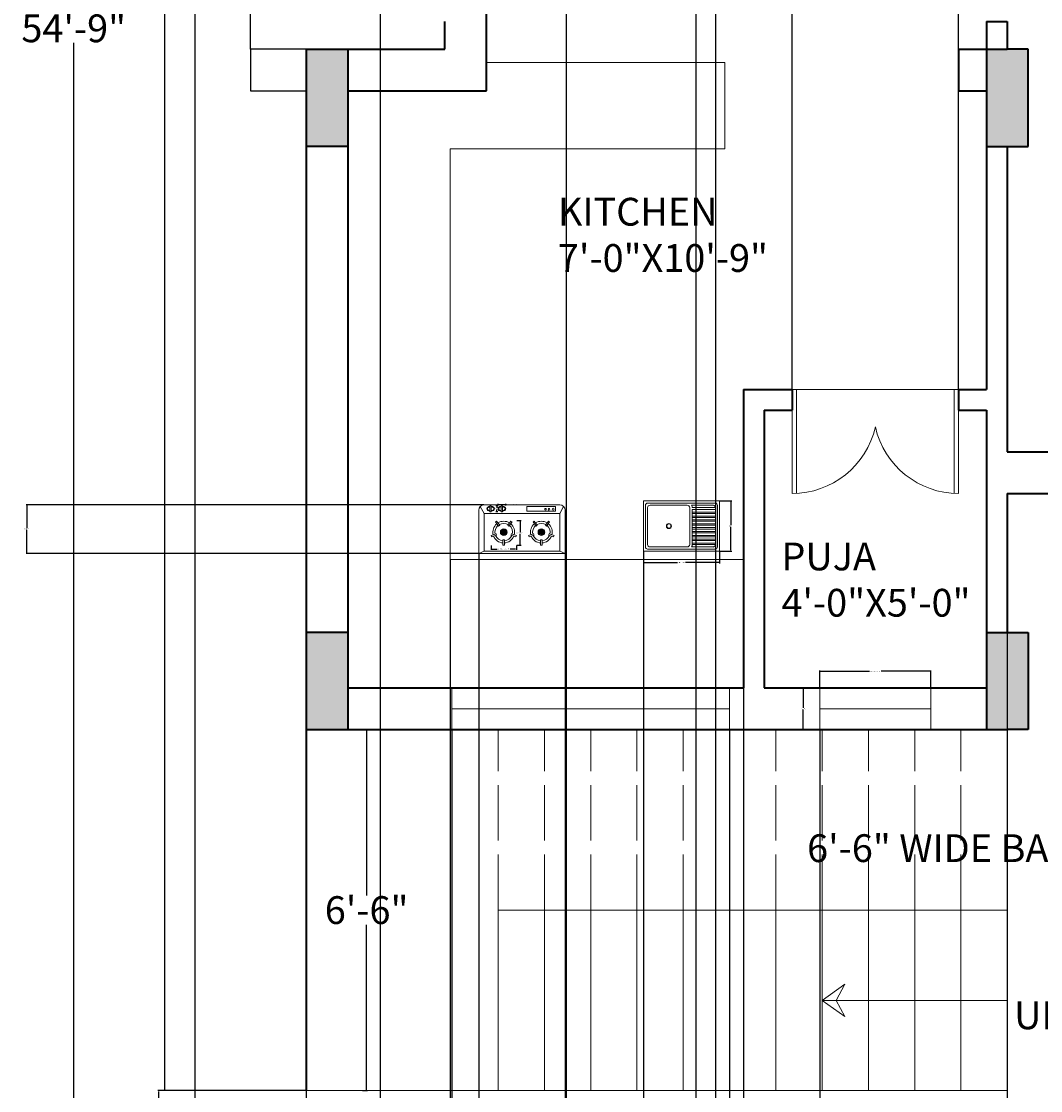
# Model space of a CAD drawing. Units: inches. Extents: x -36 to 401, y -686 to 73.
# Tile 2 of 15: x -36 to 184, y -550 to -319. Entities that reach past the tile are written whole.
import ezdxf

# ---------------------------------------------------------------- set-up
doc = ezdxf.new("R2010")
doc.units = ezdxf.units.IN
doc.header["$MEASUREMENT"] = 0
doc.linetypes.add('ACAD_ISO02W100', pattern=[15, 12, -3])
for name, color, linetype, lineweight in [('A-ANNO-DIMS', 2, 'Continuous', 18), ('A-ANNO-SYMB', 7, 'Continuous', 18), ('A-ANNO-TEXT', 7, 'Continuous', 18), ('A-AREA-IDEN', 7, 'Continuous', 18), ('A-COLS', 7, 'Continuous', 40), ('A-COLS-PATT', 22, 'Continuous', 13), ('A-DOOR', 3, 'Continuous', 18), ('A-EQPM', 8, 'Continuous', 13), ('A-FLOR', 7, 'Continuous', 25), ('A-FLOR-CASE', 9, 'Continuous', 18), ('A-FLOR-FIXT', 9, 'Continuous', 18), ('A-FLOR-OVHD', 8, 'ACAD_ISO02W100', 18), ('A-FLOR-STRS', 7, 'Continuous', 18), ('A-FLOR-STRS-OVHD', 8, 'ACAD_ISO02W100', 13), ('A-GLAZ', 4, 'Continuous', 18), ('A-WALL', 7, 'Continuous', 35), ('C-PROP', 7, 'Continuous', 25)]:
    doc.layers.add(name, color=color, linetype=linetype, lineweight=lineweight)
doc.styles.get("Standard").update_dxf_attribs({"font": 'arial.ttf'})
doc.dimstyles.get("Standard").update_dxf_attribs({"dimtxt": 0.18, "dimasz": 0.18, "dimexe": 0.18, "dimexo": 0.0625, "dimgap": 0.09, "dimtad": 0, "dimtih": 1, "dimtoh": 1, "dimdec": 0, "dimzin": 0, "dimdsep": 46, "dimlunit": 3, "dimtxsty": 'Standard', "dimcen": 0.09, "dimadec": 0, "dimazin": 0, "dimtfac": 1, "dimtdec": 0, "dimtofl": 0, "dimtmove": 0, "dimatfit": 3, "dimfxl": 1, "dimtolj": 1, "dimtzin": 0, "dimarcsym": 0})

# ---------------------------------------------------------------- blocks, each defined once
blk = doc.blocks.new('М12 540х820')
for p, q in [((0, 540), (-820, 540)), ((-820, 540), (-820, 0)), ((-798, 495), (-798, 45)), ((-45, 517), (-775, 517)), ((-775, 468), (-775, 72)), ((-348, 495), (-748, 495)), ((-320, 468), (-320, 72)), ((-302, 495), (-65, 495)), ((-294, 468), (-294, 472)), ((-294, 468), (-45, 468)), ((-45, 470), (-45, 468)), ((-22, 45), (-22, 495)), ((0, 0), (0, 540)), ((-294, 447), (-45, 447)), ((-294, 420), (-294, 447)), ((-294, 420), (-45, 420)), ((-294, 405), (-45, 405)), ((-294, 378), (-294, 405)), ((-294, 378), (-45, 378)), ((-294, 336), (-294, 363)), ((-294, 363), (-45, 363)), ((-45, 420), (-45, 447)), ((-45, 378), (-45, 405)), ((-45, 336), (-45, 363)), ((-294, 336), (-45, 336)), ((-294, 295), (-294, 322)), ((-294, 322), (-45, 322)), ((-294, 295), (-45, 295)), ((-294, 253), (-294, 280)), ((-294, 280), (-45, 280)), ((-294, 253), (-45, 253)), ((-294, 211), (-294, 238)), ((-294, 238), (-45, 238)), ((-45, 295), (-45, 322)), ((-45, 253), (-45, 280)), ((-45, 211), (-45, 238)), ((-294, 211), (-45, 211)), ((-294, 170), (-294, 197)), ((-294, 197), (-45, 197)), ((-294, 170), (-45, 170)), ((-294, 128), (-294, 155)), ((-294, 155), (-45, 155)), ((-294, 128), (-45, 128)), ((-45, 170), (-45, 197)), ((-45, 128), (-45, 155)), ((-820, 0), (0, 0)), ((-775, 22), (-45, 22)), ((-748, 45), (-348, 45)), ((-302, 45), (-65, 45)), ((-294, 114), (-45, 114)), ((-294, 87), (-294, 114)), ((-294, 87), (-45, 87)), ((-294, 72), (-45, 72)), ((-45, 87), (-45, 114)), ((-45, 70), (-45, 72))]:
    blk.add_line(p, q)
at = {"ltscale": 0.06}
for p, q in [((-820, 0), (-820, 540)), ((-820, 540), (0, 540)), ((0, 540), (0, 537)), ((0, 537), (0, 0)), ((-294, 447), (-45, 447)), ((-294, 405), (-294, 447)), ((-294, 363), (-294, 405)), ((-294, 322), (-294, 363)), ((-45, 447), (-45, 420)), ((-45, 420), (-45, 378)), ((-45, 378), (-45, 336)), ((-294, 280), (-294, 322)), ((-294, 238), (-294, 280)), ((-294, 197), (-294, 238)), ((-45, 336), (-45, 295)), ((-45, 295), (-45, 253)), ((-45, 253), (-45, 211)), ((-294, 155), (-294, 197)), ((-294, 114), (-294, 155)), ((-45, 211), (-45, 170)), ((-45, 170), (-45, 128)), ((-45, 128), (-45, 87)), ((0, 0), (-820, 0)), ((-294, 72), (-294, 114)), ((-45, 72), (-294, 72)), ((-45, 87), (-45, 72))]:
    blk.add_line(p, q, dxfattribs=at)
at = {"extrusion": (0, 0, -1)}
for centre, major_axis, start_param, end_param in [((-775, 495), (-15.9, 15.9), -0.785398, 0.785398), ((-775, 495), (-15.9, 15.9), -0.785398, 0.785398), ((-748, 468), (-19.1, -19.1), 0.785398, 2.356194), ((-748, 468), (-19.1, -19.1), 0.785398, 2.356194), ((-348, 468), (-19.1, 19.1), 0.785398, 2.356194), ((-348, 468), (-19.1, 19.1), 0.785398, 2.356194), ((-343, 468), (-35, 35), 1.779263, 2.356194), ((-343, 468), (-35, 35), 1.779263, 2.356192), ((-343, 468), (-35, 35), 2.356192, 2.356194), ((-72, 469), (-19.3, 19.3), 1.0328, 2.38382), ((-72, 469), (-19.3, 19.3), 1.0328, 1.064673), ((-72, 469), (-19.3, 19.3), 1.064673, 2.328569), ((-45, 495), (-15.9, -15.9), 2.356194, 3.926991), ((-45, 495), (-15.9, -15.9), 2.356194, 3.926991), ((-72, 469), (-19.3, 19.3), 2.328569, 2.38382), ((-545, 270), (-19.1, -19.1), 3.926991, 10.210176), ((-545, 270), (-19.1, -19.1), 3.926991, 10.210176), ((-545, 270), (-15.9, -15.9), 3.926991, 10.210176), ((-545, 270), (-15.9, -15.9), 3.926991, 10.210176), ((-775, 45), (-15.9, -15.9), 5.497787, 7.068583), ((-775, 45), (-15.9, -15.9), 5.497787, 7.068583), ((-748, 72), (-19.1, 19.1), 3.926991, 5.497787), ((-748, 72), (-19.1, 19.1), 3.926991, 5.497787), ((-348, 72), (-19.1, -19.1), 3.926991, 5.497787), ((-348, 72), (-19.1, -19.1), 3.926991, 5.497787), ((-343, 72), (-35, -35), 3.926991, 4.503922), ((-343, 72), (-35, -35), 3.926991, 4.503922), ((-72, 71), (-19.3, -19.3), 3.899365, 5.250385), ((-72, 71), (-19.3, -19.3), 5.218512, 5.250385), ((-72, 71), (-19.3, -19.3), 3.954617, 5.218512), ((-72, 71), (-19.3, -19.3), 3.899365, 3.954617), ((-45, 45), (-15.9, 15.9), 2.356194, 3.926991), ((-45, 45), (-15.9, 15.9), 2.356194, 3.926991)]:
    blk.add_ellipse(centre, major_axis=major_axis, ratio=1, start_param=start_param, end_param=end_param, dxfattribs=at)
blk = doc.blocks.new('*D2')
at = {"layer": 'A-ANNO-DIMS', "color": 0, "lineweight": -2, "transparency": 16777216}
for p, q in [((37.9, -472.21), (38.96, -472.21)), ((38.78, -472.39), (38.78, -508.06)), ((38.78, -550.03), (38.78, -514.36)), ((37.9, -550.21), (38.96, -550.21))]:
    blk.add_line(p, q, dxfattribs=at)
at = {"layer": 'A-ANNO-DIMS', "color": 0, "transparency": 16777216}
for points in [[(38.75, -472.39), (38.81, -472.39), (38.78, -472.21)], [(38.75, -550.03), (38.81, -550.03), (38.78, -550.21)]]:
    blk.add_solid(points, dxfattribs=at)
at = {"layer": 'Defpoints', "color": 0, "transparency": 16777216}
for p in [(37.84, -472.21), (38.78, -472.21), (37.84, -550.21)]:
    blk.add_point(p, dxfattribs=at)
at = {"layer": 'A-ANNO-DIMS', "color": 0, "transparency": 16777216, "insert": (38.78, -511.21), "char_height": 6, "attachment_point": 5}
blk.add_mtext('\\A1;6\'-6"', dxfattribs=at)
blk = doc.blocks.new('*D8')
at = {"layer": 'A-ANNO-DIMS', "color": 0, "lineweight": -2, "transparency": 16777216}
for p, q in [((25.63, 7.79), (-24.68, 7.79)), ((-24.5, 7.61), (-24.5, -317.56)), ((-24.5, -649.03), (-24.5, -323.86)), ((1.63, -649.21), (-24.68, -649.21))]:
    blk.add_line(p, q, dxfattribs=at)
at = {"layer": 'A-ANNO-DIMS', "color": 0, "transparency": 16777216}
for points in [[(-24.53, 7.61), (-24.47, 7.61), (-24.5, 7.79)], [(-24.53, -649.03), (-24.47, -649.03), (-24.5, -649.21)]]:
    blk.add_solid(points, dxfattribs=at)
at = {"layer": 'Defpoints', "color": 0, "transparency": 16777216}
for p in [(25.69, 7.79), (-24.5, -649.21), (1.69, -649.21)]:
    blk.add_point(p, dxfattribs=at)
at = {"layer": 'A-ANNO-DIMS', "color": 0, "transparency": 16777216, "insert": (-24.5, -320.71), "char_height": 6, "attachment_point": 5}
blk.add_mtext('\\A1;54\'-9"', dxfattribs=at)
blk = doc.blocks.new('*D11')
at = {"layer": 'A-ANNO-DIMS', "color": 0, "lineweight": -2, "transparency": 16777216}
for p, q in [((25.63, 7.79), (-5.02, 7.79)), ((-4.84, 7.61), (-4.84, -268.06)), ((-4.84, -550.03), (-4.84, -274.36)), ((25.63, -550.21), (-5.02, -550.21))]:
    blk.add_line(p, q, dxfattribs=at)
at = {"layer": 'A-ANNO-DIMS', "color": 0, "transparency": 16777216}
for points in [[(-4.87, 7.61), (-4.81, 7.61), (-4.84, 7.79)], [(-4.87, -550.03), (-4.81, -550.03), (-4.84, -550.21)]]:
    blk.add_solid(points, dxfattribs=at)
at = {"layer": 'Defpoints', "color": 0, "transparency": 16777216}
for p in [(25.69, 7.79), (-4.84, -550.21), (25.69, -550.21)]:
    blk.add_point(p, dxfattribs=at)
at = {"layer": 'A-ANNO-DIMS', "color": 0, "transparency": 16777216, "insert": (-4.84, -271.21), "char_height": 6, "attachment_point": 5}
blk.add_mtext('\\A1;46\'-6"', dxfattribs=at)
blk = doc.blocks.new('*D12')
at = {"layer": 'A-ANNO-DIMS', "color": 0, "lineweight": -2, "transparency": 16777216}
for p, q in [((25.63, -550.21), (-6.34, -550.21)), ((-6.16, -550.39), (-6.16, -596.55)), ((-6.16, -649.03), (-6.16, -602.87)), ((25.63, -649.21), (-6.34, -649.21))]:
    blk.add_line(p, q, dxfattribs=at)
at = {"layer": 'A-ANNO-DIMS', "color": 0, "transparency": 16777216}
for points in [[(-6.19, -550.39), (-6.13, -550.39), (-6.16, -550.21)], [(-6.19, -649.03), (-6.13, -649.03), (-6.16, -649.21)]]:
    blk.add_solid(points, dxfattribs=at)
at = {"layer": 'Defpoints', "color": 0, "transparency": 16777216}
for p in [(25.69, -550.21), (-6.16, -649.21), (25.69, -649.21)]:
    blk.add_point(p, dxfattribs=at)
at = {"layer": 'A-ANNO-DIMS', "color": 0, "transparency": 16777216, "insert": (-6.16, -599.71), "char_height": 6, "attachment_point": 5}
blk.add_mtext('\\A1;8\'-3"', dxfattribs=at)
blk = doc.blocks.new('WIN-24IN')
for p, q in [((0, 9), (24, 9)), ((0, 0), (0, 9)), ((24, 9), (24, 0)), ((0, 4.5), (24, 4.5)), ((24, 0), (0, 0))]:
    blk.add_line(p, q)
blk = doc.blocks.new('WIN-60IN')
for p, q in [((0, 9), (60, 9)), ((0, 0), (0, 9)), ((60, 9), (60, 0)), ((0, 4.5), (60, 4.5)), ((60, 0), (0, 0))]:
    blk.add_line(p, q)
blk = doc.blocks.new('HOB-BURNER')
for p, q in [((0.95, 5.03), (1.21, 5.22)), ((1.62, 4.11), (0.95, 5.03)), ((1.21, 5.22), (1.87, 4.3)), ((3.61, 4.3), (4.28, 5.22)), ((4.54, 5.03), (3.87, 4.11)), ((4.28, 5.22), (4.54, 5.03)), ((0, 2.11), (1.08, 2.46)), ((1.08, 2.46), (1.18, 2.16)), ((1.87, 4.3), (1.62, 4.11)), ((2.74, 2.83), (2.02, 2.83)), ((2.74, 2.83), (2.06, 3.05)), ((2.74, 2.83), (2.06, 2.61)), ((2.74, 2.83), (2.16, 3.25)), ((2.74, 2.83), (2.16, 2.41)), ((2.74, 2.83), (2.32, 3.41)), ((2.74, 2.83), (2.32, 2.25)), ((2.74, 2.83), (2.52, 3.51)), ((2.74, 2.83), (2.52, 2.15)), ((2.74, 2.83), (2.74, 3.55)), ((2.74, 2.83), (2.97, 3.51)), ((2.74, 2.83), (3.17, 3.41)), ((2.74, 2.83), (3.32, 3.25)), ((2.74, 2.83), (3.43, 3.05)), ((2.74, 2.83), (3.46, 2.83)), ((2.74, 2.83), (3.43, 2.61)), ((2.74, 2.83), (3.32, 2.41)), ((2.74, 2.83), (3.17, 2.25)), ((2.74, 2.83), (2.97, 2.15)), ((2.74, 2.83), (2.74, 2.11)), ((3.87, 4.11), (3.61, 4.3)), ((4.31, 2.16), (4.41, 2.46)), ((4.41, 2.46), (5.49, 2.11)), ((0.1, 1.81), (0, 2.11)), ((1.18, 2.16), (0.1, 1.81)), ((2.58, 1.13), (2.9, 1.13)), ((2.58, 0), (2.58, 1.13)), ((2.9, 1.13), (2.9, 0)), ((5.39, 1.81), (4.31, 2.16)), ((5.49, 2.11), (5.39, 1.81)), ((2.9, 0), (2.58, 0))]:
    blk.add_line(p, q)
blk.add_circle((2.74, 2.83), 0.721)
for radius, start, end in [(2.35, 129.8765, 194.1235), (2.35, 57.8765, 122.1235), (1.89, 58.8365, 121.1635), (2.35, 345.8765, 50.1235), (1.89, 130.8365, 193.1635), (1.89, 346.8365, 49.1635), (2.35, 201.8765, 266.1235), (1.89, 202.8365, 265.1635), (1.89, 274.8365, 337.1635), (2.35, 273.8765, 338.1235)]:
    blk.add_arc((2.74, 2.83), radius, start, end)
blk = doc.blocks.new('HOB-CONTROL')
for p, q in [((0.67, 0), (0.67, 1.29)), ((0.67, 1.29), (0.97, 1.29)), ((0.97, 1.29), (0.97, 0)), ((0.97, 0), (0.67, 0))]:
    blk.add_line(p, q)
for major_axis, start_param, end_param in [((0.835, 0), 1.774361, 4.508825), ((-0.835, 0), 1.73081, 4.552375)]:
    blk.add_ellipse((0.84, 0.65), major_axis=major_axis, ratio=0.671641, start_param=start_param, end_param=end_param)
for points, knots in [([(0.67, 1.08), (0.63, 1.08), (0.59, 1.07), (0.5, 1.04), (0.45, 1.03), (0.36, 0.98), (0.32, 0.96), (0.25, 0.91), (0.23, 0.88), (0.18, 0.83), (0.16, 0.8), (0.13, 0.74), (0.12, 0.71), (0.12, 0.66), (0.12, 0.63), (0.13, 0.57), (0.14, 0.54), (0.17, 0.49), (0.19, 0.46), (0.24, 0.4), (0.27, 0.38), (0.35, 0.33), (0.39, 0.31), (0.48, 0.27), (0.52, 0.25), (0.61, 0.23), (0.64, 0.22), (0.67, 0.22)], [8.079302, 8.079302, 8.079302, 8.079302, 8.245651, 8.245651, 8.463703, 8.463703, 8.681755, 8.681755, 8.899807, 8.899807, 9.117859, 9.117859, 9.33591, 9.33591, 9.553962, 9.553962, 9.772014, 9.772014, 9.990066, 9.990066, 10.208118, 10.208118, 10.426169, 10.426169, 10.644221, 10.644221, 10.770253, 10.770253, 10.770253, 10.770253]), ([(0.97, 0.21), (1, 0.22), (1.03, 0.22), (1.11, 0.24), (1.16, 0.26), (1.25, 0.29), (1.3, 0.31), (1.37, 0.36), (1.41, 0.39), (1.47, 0.44), (1.49, 0.47), (1.52, 0.52), (1.54, 0.55), (1.55, 0.61), (1.55, 0.63), (1.55, 0.65), (1.55, 0.68), (1.55, 0.71), (1.53, 0.76), (1.52, 0.79), (1.48, 0.85), (1.45, 0.88), (1.39, 0.93), (1.35, 0.96), (1.27, 1), (1.23, 1.02), (1.13, 1.05), (1.08, 1.07), (1.01, 1.08), (0.99, 1.08), (0.97, 1.09)], [4.889299, 4.889299, 4.889299, 4.889299, 5.015191, 5.015191, 5.233243, 5.233243, 5.451295, 5.451295, 5.669347, 5.669347, 5.887399, 5.887399, 6.10545, 6.10545, 6.283185, 6.283185, 6.283185, 6.501237, 6.501237, 6.719289, 6.719289, 6.937341, 6.937341, 7.155392, 7.155392, 7.373444, 7.373444, 7.591496, 7.591496, 7.677072, 7.677072, 7.677072, 7.677072])]:
    blk.add_open_spline(points, degree=3, knots=knots)
blk = doc.blocks.new('*D39')
at = {"layer": 'A-ANNO-DIMS', "color": 0, "lineweight": -2, "transparency": 16777216}
for p, q in [((136.69, -463.15), (136.69, -459.43)), ((136.87, -459.61), (147.46, -459.61)), ((160.51, -459.61), (149.92, -459.61)), ((160.69, -463.15), (160.69, -459.43))]:
    blk.add_line(p, q, dxfattribs=at)
at = {"layer": 'A-ANNO-DIMS', "color": 0, "transparency": 16777216}
for points in [[(136.87, -459.58), (136.87, -459.64), (136.69, -459.61)], [(160.51, -459.58), (160.51, -459.64), (160.69, -459.61)]]:
    blk.add_solid(points, dxfattribs=at)
at = {"layer": 'Defpoints', "color": 0, "transparency": 16777216}
for p in [(160.69, -459.61), (136.69, -463.21), (160.69, -463.21)]:
    blk.add_point(p, dxfattribs=at)
at = {"layer": 'A-ANNO-DIMS', "color": 0, "transparency": 16777216, "insert": (148.69, -459.61), "char_height": 0.18, "attachment_point": 5}
blk.add_mtext('\\A1;WINDOW 2\'-0" TYP.', dxfattribs=at)
blk = doc.blocks.new('*D40')
at = {"layer": 'A-ANNO-DIMS', "color": 0, "lineweight": -2, "transparency": 16777216}
for p, q in [((136.63, -463.21), (132.91, -463.21)), ((133.09, -463.39), (133.09, -467.53)), ((133.09, -472.03), (133.09, -467.89)), ((136.63, -472.21), (132.91, -472.21))]:
    blk.add_line(p, q, dxfattribs=at)
at = {"layer": 'A-ANNO-DIMS', "color": 0, "transparency": 16777216}
for points in [[(133.06, -463.39), (133.12, -463.39), (133.09, -463.21)], [(133.06, -472.03), (133.12, -472.03), (133.09, -472.21)]]:
    blk.add_solid(points, dxfattribs=at)
at = {"layer": 'Defpoints', "color": 0, "transparency": 16777216}
for p in [(133.09, -463.21), (136.69, -463.21), (136.69, -472.21)]:
    blk.add_point(p, dxfattribs=at)
at = {"layer": 'A-ANNO-DIMS', "color": 0, "transparency": 16777216, "insert": (133.09, -467.71), "char_height": 0.18, "attachment_point": 5}
blk.add_mtext('\\A1;0\'-9" TYP.', dxfattribs=at)
blk = doc.blocks.new('*D53')
at = {"layer": 'A-ANNO-DIMS', "color": 0, "lineweight": -2, "transparency": 16777216}
for p, q in [((65.66, -432.44), (65.66, -433.38)), ((65.84, -433.2), (67, -433.2)), ((70.97, -433.2), (69.82, -433.2)), ((71.15, -432.44), (71.15, -433.38))]:
    blk.add_line(p, q, dxfattribs=at)
at = {"layer": 'A-ANNO-DIMS', "color": 0, "transparency": 16777216}
for points in [[(65.84, -433.17), (65.84, -433.23), (65.66, -433.2)], [(70.97, -433.17), (70.97, -433.23), (71.15, -433.2)]]:
    blk.add_solid(points, dxfattribs=at)
at = {"layer": 'Defpoints', "color": 0, "transparency": 16777216}
for p in [(65.66, -432.38), (71.15, -432.38), (71.15, -433.2)]:
    blk.add_point(p, dxfattribs=at)
at = {"layer": 'A-ANNO-DIMS', "color": 0, "transparency": 16777216, "insert": (68.41, -433.2), "char_height": 0.18, "attachment_point": 5}
blk.add_mtext('\\A1;BURNER 0\'-5 1/2" TYP.', dxfattribs=at)
blk = doc.blocks.new('*D54')
at = {"layer": 'A-ANNO-DIMS', "color": 0, "lineweight": -2, "transparency": 16777216}
for p, q in [((71.21, -427.07), (72.15, -427.07)), ((71.97, -427.25), (71.97, -429.54)), ((71.97, -432.2), (71.97, -429.91)), ((71.21, -432.38), (72.15, -432.38))]:
    blk.add_line(p, q, dxfattribs=at)
at = {"layer": 'A-ANNO-DIMS', "color": 0, "transparency": 16777216}
for points in [[(71.94, -427.25), (72, -427.25), (71.97, -427.07)], [(71.94, -432.2), (72, -432.2), (71.97, -432.38)]]:
    blk.add_solid(points, dxfattribs=at)
at = {"layer": 'Defpoints', "color": 0, "transparency": 16777216}
for p in [(71.15, -427.07), (71.97, -427.07), (71.15, -432.38)]:
    blk.add_point(p, dxfattribs=at)
at = {"layer": 'A-ANNO-DIMS', "color": 0, "transparency": 16777216, "insert": (71.97, -429.73), "char_height": 0.18, "attachment_point": 5}
blk.add_mtext('\\A1;0\'-5 1/2" TYP.', dxfattribs=at)
blk = doc.blocks.new('*D55')
at = {"layer": 'A-ANNO-DIMS', "color": 0, "lineweight": -2, "transparency": 16777216}
for p, q in [((67.17, -423.79), (67.17, -423.43)), ((67.35, -423.61), (68.65, -423.61)), ((68.83, -423.79), (68.83, -423.43)), ((68.83, -423.61), (69.01, -423.61))]:
    blk.add_line(p, q, dxfattribs=at)
at = {"layer": 'A-ANNO-DIMS', "color": 0, "transparency": 16777216}
for points in [[(67.35, -423.58), (67.35, -423.64), (67.17, -423.61)], [(68.65, -423.58), (68.65, -423.64), (68.83, -423.61)]]:
    blk.add_solid(points, dxfattribs=at)
at = {"layer": 'Defpoints', "color": 0, "transparency": 16777216}
for p in [(67.17, -423.86), (68.83, -423.61), (68.83, -423.86)]:
    blk.add_point(p, dxfattribs=at)
at = {"layer": 'A-ANNO-DIMS', "color": 0, "transparency": 16777216, "insert": (70.51, -423.61), "char_height": 0.18, "attachment_point": 5}
blk.add_mtext('\\A1;CONTROL 0\'-1 1/2" TYP.', dxfattribs=at)
blk = doc.blocks.new('*D56')
at = {"layer": 'A-ANNO-DIMS', "color": 0, "lineweight": -2, "transparency": 16777216}
for p, q in [((67.1, -423.86), (66.73, -423.86)), ((66.91, -424.04), (66.91, -424.32)), ((66.91, -424.97), (66.91, -424.69)), ((67.1, -425.15), (66.73, -425.15))]:
    blk.add_line(p, q, dxfattribs=at)
at = {"layer": 'A-ANNO-DIMS', "color": 0, "transparency": 16777216}
for points in [[(66.88, -424.04), (66.94, -424.04), (66.91, -423.86)], [(66.88, -424.97), (66.94, -424.97), (66.91, -425.15)]]:
    blk.add_solid(points, dxfattribs=at)
at = {"layer": 'Defpoints', "color": 0, "transparency": 16777216}
for p in [(66.91, -423.86), (67.17, -423.86), (67.17, -425.15)]:
    blk.add_point(p, dxfattribs=at)
at = {"layer": 'A-ANNO-DIMS', "color": 0, "transparency": 16777216, "insert": (66.91, -424.5), "char_height": 0.18, "attachment_point": 5}
blk.add_mtext('\\A1;0\'-1 1/2" TYP.', dxfattribs=at)
blk = doc.blocks.new('*D61')
at = {"layer": 'A-ANNO-DIMS', "color": 0, "lineweight": -2, "transparency": 16777216}
for p, q in [((98.57, -433.72), (98.57, -436.31)), ((115.03, -433.72), (115.03, -436.31)), ((98.75, -436.13), (105.93, -436.13)), ((114.85, -436.13), (107.66, -436.13))]:
    blk.add_line(p, q, dxfattribs=at)
at = {"layer": 'A-ANNO-DIMS', "color": 0, "transparency": 16777216}
for points in [[(98.75, -436.1), (98.75, -436.16), (98.57, -436.13)], [(114.85, -436.1), (114.85, -436.16), (115.03, -436.13)]]:
    blk.add_solid(points, dxfattribs=at)
at = {"layer": 'Defpoints', "color": 0, "transparency": 16777216}
for p in [(98.57, -433.66), (115.03, -433.66), (115.03, -436.13)]:
    blk.add_point(p, dxfattribs=at)
at = {"layer": 'A-ANNO-DIMS', "color": 0, "transparency": 16777216, "insert": (106.8, -436.13), "char_height": 0.18, "attachment_point": 5}
blk.add_mtext('\\A1;SINK 1\'-4 1/2"', dxfattribs=at)
blk = doc.blocks.new('*D62')
at = {"layer": 'A-ANNO-DIMS', "color": 0, "lineweight": -2, "transparency": 16777216}
for p, q in [((115.09, -422.82), (117.67, -422.82)), ((117.49, -423), (117.49, -428.06)), ((117.49, -433.48), (117.49, -428.42)), ((115.09, -433.66), (117.67, -433.66))]:
    blk.add_line(p, q, dxfattribs=at)
at = {"layer": 'A-ANNO-DIMS', "color": 0, "transparency": 16777216}
for points in [[(117.46, -423), (117.52, -423), (117.49, -422.82)], [(117.46, -433.48), (117.52, -433.48), (117.49, -433.66)]]:
    blk.add_solid(points, dxfattribs=at)
at = {"layer": 'Defpoints', "color": 0, "transparency": 16777216}
for p in [(115.03, -422.82), (117.49, -422.82), (115.03, -433.66)]:
    blk.add_point(p, dxfattribs=at)
at = {"layer": 'A-ANNO-DIMS', "color": 0, "transparency": 16777216, "insert": (117.49, -428.24), "char_height": 0.18, "attachment_point": 5}
blk.add_mtext('\\A1;0\'-11"', dxfattribs=at)
blk = doc.blocks.new('*D73')
at = {"layer": 'A-ANNO-DIMS', "color": 0, "lineweight": -2, "transparency": 16777216}
for p, q in [((177.19, -421.27), (177.19, -685.69)), ((253.69, -421.27), (253.69, -685.69)), ((177.37, -685.51), (214.9, -685.51)), ((253.51, -685.51), (215.98, -685.51))]:
    blk.add_line(p, q, dxfattribs=at)
at = {"layer": 'A-ANNO-DIMS', "color": 0, "transparency": 16777216}
for points in [[(177.37, -685.48), (177.37, -685.54), (177.19, -685.51)], [(253.51, -685.48), (253.51, -685.54), (253.69, -685.51)]]:
    blk.add_solid(points, dxfattribs=at)
at = {"layer": 'Defpoints', "color": 0, "transparency": 16777216}
for p in [(177.19, -421.21), (253.69, -421.21), (253.69, -685.51)]:
    blk.add_point(p, dxfattribs=at)
at = {"layer": 'A-ANNO-DIMS', "color": 0, "transparency": 16777216, "insert": (215.44, -685.51), "char_height": 0.18, "attachment_point": 5}
blk.add_mtext('\\A1;6\'-4 1/2"', dxfattribs=at)
blk = doc.blocks.new('*D75')
at = {"layer": 'A-ANNO-DIMS', "color": 0, "lineweight": -2, "transparency": 16777216}
for p, q in [((25.69, -472.27), (25.69, -685.69)), ((57.17, -472.27), (57.17, -685.69)), ((25.87, -685.51), (40.89, -685.51)), ((56.99, -685.51), (41.97, -685.51))]:
    blk.add_line(p, q, dxfattribs=at)
at = {"layer": 'A-ANNO-DIMS', "color": 0, "transparency": 16777216}
for points in [[(25.87, -685.48), (25.87, -685.54), (25.69, -685.51)], [(56.99, -685.48), (56.99, -685.54), (57.17, -685.51)]]:
    blk.add_solid(points, dxfattribs=at)
at = {"layer": 'Defpoints', "color": 0, "transparency": 16777216}
for p in [(25.69, -472.21), (57.17, -472.21), (57.17, -685.51)]:
    blk.add_point(p, dxfattribs=at)
at = {"layer": 'A-ANNO-DIMS', "color": 0, "transparency": 16777216, "insert": (41.43, -685.51), "char_height": 0.18, "attachment_point": 5}
blk.add_mtext('\\A1;2\'-7 1/2"', dxfattribs=at)
blk = doc.blocks.new('*D76')
at = {"layer": 'A-ANNO-DIMS', "color": 0, "lineweight": -2, "transparency": 16777216}
for p, q in [((117.19, -472.27), (117.19, -685.69)), ((136.69, -472.27), (136.69, -685.69)), ((117.37, -685.51), (126.41, -685.51)), ((136.51, -685.51), (127.47, -685.51))]:
    blk.add_line(p, q, dxfattribs=at)
at = {"layer": 'A-ANNO-DIMS', "color": 0, "transparency": 16777216}
for points in [[(117.37, -685.48), (117.37, -685.54), (117.19, -685.51)], [(136.51, -685.48), (136.51, -685.54), (136.69, -685.51)]]:
    blk.add_solid(points, dxfattribs=at)
at = {"layer": 'Defpoints', "color": 0, "transparency": 16777216}
for p in [(117.19, -472.21), (136.69, -472.21), (136.69, -685.51)]:
    blk.add_point(p, dxfattribs=at)
at = {"layer": 'A-ANNO-DIMS', "color": 0, "transparency": 16777216, "insert": (126.94, -685.51), "char_height": 0.18, "attachment_point": 5}
blk.add_mtext('\\A1;1\'-7 1/2"', dxfattribs=at)
blk = doc.blocks.new('*D79')
at = {"layer": 'A-ANNO-DIMS', "color": 0, "lineweight": -2, "transparency": 16777216}
for p, q in [((130.69, -398.65), (130.69, 68.27)), ((130.87, 68.09), (148.36, 68.09)), ((166.51, 68.09), (149.02, 68.09)), ((166.69, -398.65), (166.69, 68.27))]:
    blk.add_line(p, q, dxfattribs=at)
at = {"layer": 'A-ANNO-DIMS', "color": 0, "transparency": 16777216}
for points in [[(130.87, 68.12), (130.87, 68.06), (130.69, 68.09)], [(166.51, 68.12), (166.51, 68.06), (166.69, 68.09)]]:
    blk.add_solid(points, dxfattribs=at)
at = {"layer": 'Defpoints', "color": 0, "transparency": 16777216}
for p in [(166.69, 68.09), (130.69, -398.71), (166.69, -398.71)]:
    blk.add_point(p, dxfattribs=at)
at = {"layer": 'A-ANNO-DIMS', "color": 0, "transparency": 16777216, "insert": (148.69, 68.09), "char_height": 0.18, "attachment_point": 5}
blk.add_mtext('\\A1;3\'-0"', dxfattribs=at)
blk = doc.blocks.new('*D80')
at = {"layer": 'A-ANNO-DIMS', "color": 0, "lineweight": -2, "transparency": 16777216}
for p, q in [((56.84, -435.52), (56.84, -685.69)), ((120.19, -435.52), (120.19, -685.69)), ((57.02, -685.51), (87.97, -685.51)), ((120.01, -685.51), (89.05, -685.51))]:
    blk.add_line(p, q, dxfattribs=at)
at = {"layer": 'A-ANNO-DIMS', "color": 0, "transparency": 16777216}
for points in [[(57.02, -685.48), (57.02, -685.54), (56.84, -685.51)], [(120.01, -685.48), (120.01, -685.54), (120.19, -685.51)]]:
    blk.add_solid(points, dxfattribs=at)
at = {"layer": 'Defpoints', "color": 0, "transparency": 16777216}
for p in [(56.84, -435.46), (120.19, -435.46), (120.19, -685.51)]:
    blk.add_point(p, dxfattribs=at)
at = {"layer": 'A-ANNO-DIMS', "color": 0, "transparency": 16777216, "insert": (88.51, -685.51), "char_height": 0.18, "attachment_point": 5}
blk.add_mtext('\\A1;5\'-3 1/2"', dxfattribs=at)
blk = doc.blocks.new('*D81')
at = {"layer": 'A-ANNO-DIMS', "color": 0, "lineweight": -2, "transparency": 16777216}
for p, q in [((63, -434.2), (63, -685.69)), ((81.66, -434.2), (81.66, -685.69)), ((63.18, -685.51), (71.8, -685.51)), ((81.48, -685.51), (72.86, -685.51))]:
    blk.add_line(p, q, dxfattribs=at)
at = {"layer": 'A-ANNO-DIMS', "color": 0, "transparency": 16777216}
for points in [[(63.18, -685.48), (63.18, -685.54), (63, -685.51)], [(81.48, -685.48), (81.48, -685.54), (81.66, -685.51)]]:
    blk.add_solid(points, dxfattribs=at)
at = {"layer": 'Defpoints', "color": 0, "transparency": 16777216}
for p in [(63, -434.14), (81.66, -434.14), (81.66, -685.51)]:
    blk.add_point(p, dxfattribs=at)
at = {"layer": 'A-ANNO-DIMS', "color": 0, "transparency": 16777216, "insert": (72.33, -685.51), "char_height": 0.18, "attachment_point": 5}
blk.add_mtext('\\A1;1\'-6 1/2"', dxfattribs=at)
blk = doc.blocks.new('*D82')
at = {"layer": 'A-ANNO-DIMS', "color": 0, "lineweight": -2, "transparency": 16777216}
for p, q in [((64.1, -423.65), (-34.79, -423.65)), ((-34.61, -423.83), (-34.61, -428.71)), ((-34.61, -433.96), (-34.61, -429.08)), ((62.94, -434.14), (-34.79, -434.14))]:
    blk.add_line(p, q, dxfattribs=at)
at = {"layer": 'A-ANNO-DIMS', "color": 0, "transparency": 16777216}
for points in [[(-34.64, -423.83), (-34.58, -423.83), (-34.61, -423.65)], [(-34.64, -433.96), (-34.58, -433.96), (-34.61, -434.14)]]:
    blk.add_solid(points, dxfattribs=at)
at = {"layer": 'Defpoints', "color": 0, "transparency": 16777216}
for p in [(64.17, -423.65), (-34.61, -434.14), (63, -434.14)]:
    blk.add_point(p, dxfattribs=at)
at = {"layer": 'A-ANNO-DIMS', "color": 0, "transparency": 16777216, "insert": (-34.61, -428.89), "char_height": 0.18, "attachment_point": 5}
blk.add_mtext('\\A1;0\'-10 1/2"', dxfattribs=at)
blk = doc.blocks.new('*D83')
at = {"layer": 'A-ANNO-DIMS', "color": 0, "lineweight": -2, "transparency": 16777216}
for p, q in [((63, -434.2), (63, -685.69)), ((56.84, -435.52), (56.84, -685.69)), ((57.02, -685.51), (59.59, -685.51)), ((62.82, -685.51), (60.25, -685.51))]:
    blk.add_line(p, q, dxfattribs=at)
at = {"layer": 'A-ANNO-DIMS', "color": 0, "transparency": 16777216}
for points in [[(57.02, -685.48), (57.02, -685.54), (56.84, -685.51)], [(62.82, -685.48), (62.82, -685.54), (63, -685.51)]]:
    blk.add_solid(points, dxfattribs=at)
at = {"layer": 'Defpoints', "color": 0, "transparency": 16777216}
for p in [(63, -434.14), (56.84, -435.46), (63, -685.51)]:
    blk.add_point(p, dxfattribs=at)
at = {"layer": 'A-ANNO-DIMS', "color": 0, "transparency": 16777216, "insert": (59.92, -685.51), "char_height": 0.18, "attachment_point": 5}
blk.add_mtext('\\A1;0\'-6"', dxfattribs=at)
blk = doc.blocks.new('*D84')
at = {"layer": 'A-ANNO-DIMS', "color": 0, "lineweight": -2, "transparency": 16777216}
for p, q in [((81.66, -434.2), (81.66, -685.69)), ((98.57, -433.72), (98.57, -685.69)), ((81.84, -685.51), (89.79, -685.51)), ((98.39, -685.51), (90.43, -685.51))]:
    blk.add_line(p, q, dxfattribs=at)
at = {"layer": 'A-ANNO-DIMS', "color": 0, "transparency": 16777216}
for points in [[(81.84, -685.48), (81.84, -685.54), (81.66, -685.51)], [(98.39, -685.48), (98.39, -685.54), (98.57, -685.51)]]:
    blk.add_solid(points, dxfattribs=at)
at = {"layer": 'Defpoints', "color": 0, "transparency": 16777216}
for p in [(81.66, -434.14), (98.57, -433.66), (98.57, -685.51)]:
    blk.add_point(p, dxfattribs=at)
at = {"layer": 'A-ANNO-DIMS', "color": 0, "transparency": 16777216, "insert": (90.11, -685.51), "char_height": 0.18, "attachment_point": 5}
blk.add_mtext('\\A1;1\'-5"', dxfattribs=at)
blk = doc.blocks.new('*D85')
at = {"layer": 'A-ANNO-DIMS', "color": 0, "lineweight": -2, "transparency": 16777216}
for p, q in [((114.18, -126.31), (114.18, -685.69)), ((41.7, -137.56), (41.7, -685.69)), ((41.88, -685.51), (77.4, -685.51)), ((114, -685.51), (78.48, -685.51))]:
    blk.add_line(p, q, dxfattribs=at)
at = {"layer": 'A-ANNO-DIMS', "color": 0, "transparency": 16777216}
for points in [[(41.88, -685.48), (41.88, -685.54), (41.7, -685.51)], [(114, -685.48), (114, -685.54), (114.18, -685.51)]]:
    blk.add_solid(points, dxfattribs=at)
at = {"layer": 'Defpoints', "color": 0, "transparency": 16777216}
for p in [(114.18, -126.25), (41.7, -137.5), (114.18, -685.51)]:
    blk.add_point(p, dxfattribs=at)
at = {"layer": 'A-ANNO-DIMS', "color": 0, "transparency": 16777216, "insert": (77.94, -685.51), "char_height": 0.18, "attachment_point": 5}
blk.add_mtext('\\A1;6\'-0 1/2"', dxfattribs=at)
blk = doc.blocks.new('*D89')
at = {"layer": 'A-ANNO-DIMS', "color": 0, "lineweight": -2, "transparency": 16777216}
for p, q in [((81.9, -256.42), (81.9, -685.69)), ((109.9, -256.42), (109.9, -685.69)), ((82.08, -685.51), (95.57, -685.51)), ((109.72, -685.51), (96.23, -685.51))]:
    blk.add_line(p, q, dxfattribs=at)
at = {"layer": 'A-ANNO-DIMS', "color": 0, "transparency": 16777216}
for points in [[(82.08, -685.48), (82.08, -685.54), (81.9, -685.51)], [(109.72, -685.48), (109.72, -685.54), (109.9, -685.51)]]:
    blk.add_solid(points, dxfattribs=at)
at = {"layer": 'Defpoints', "color": 0, "transparency": 16777216}
for p in [(81.9, -256.36), (109.9, -256.36), (109.9, -685.51)]:
    blk.add_point(p, dxfattribs=at)
at = {"layer": 'A-ANNO-DIMS', "color": 0, "transparency": 16777216, "insert": (95.9, -685.51), "char_height": 0.18, "attachment_point": 5}
blk.add_mtext('\\A1;2\'-4"', dxfattribs=at)

msp = doc.modelspace()

# ---------------------------------------------------------------- hatches: boundary and pattern name
at = {"layer": 'A-COLS-PATT'}
h = msp.add_hatch(color=256, dxfattribs=at)
h.dxf.hatch_style = 1
h.paths.add_polyline_path([(34.69, 7.79), (25.69, 7.79), (25.69, -13.21), (34.69, -13.21)])
h.paths.add_polyline_path([(172.69, -13.21), (177.19, -13.21), (181.69, -13.21), (181.69, 7.79), (172.69, 7.79)])
h.paths.add_polyline_path([(322.69, 7.79), (313.69, 7.79), (313.69, -13.21), (322.69, -13.21)])
h.paths.add_polyline_path([(322.69, -157.21), (313.69, -157.21), (313.69, -178.21), (322.69, -178.21)])
h.paths.add_polyline_path([(172.69, -178.21), (177.19, -178.21), (181.69, -178.21), (181.69, -157.21), (177.19, -157.21), (172.69, -157.21)])
h.paths.add_polyline_path([(25.69, -178.21), (34.69, -178.21), (34.69, -157.21), (25.69, -157.21)])
h.paths.add_polyline_path([(34.69, -325.21), (25.69, -325.21), (25.69, -346.21), (34.69, -346.21)])
h.paths.add_polyline_path([(181.69, -325.21), (177.19, -325.21), (172.69, -325.21), (172.69, -346.21), (177.19, -346.21), (181.69, -346.21)])
h.paths.add_polyline_path([(322.69, -325.21), (313.69, -325.21), (313.69, -346.21), (322.69, -346.21)])
h.paths.add_polyline_path([(364.69, -451.21), (358.69, -451.21), (358.69, -472.21), (364.69, -472.21)])
h.paths.add_polyline_path([(181.69, -451.21), (177.19, -451.21), (172.69, -451.21), (172.69, -472.21), (177.19, -472.21), (181.69, -472.21)])
h.paths.add_polyline_path([(25.69, -472.21), (34.69, -472.21), (34.69, -451.21), (25.69, -451.21)])

# ---------------------------------------------------------------- linework, layer by layer
at = {"layer": 'A-ANNO-SYMB'}
for p, q in [((137.19, -530.71), (142.12, -527.23)), ((142.12, -527.23), (140.2, -530.71)), ((177.19, -530.71), (137.19, -530.71)), ((137.19, -530.71), (142.12, -534.19)), ((142.12, -534.19), (140.2, -530.71))]:
    msp.add_line(p, q, dxfattribs=at)
at = {"layer": 'A-COLS'}
for p, q in [((181.69, -325.21), (177.19, -325.21)), ((181.69, -346.21), (181.69, -325.21)), ((34.69, -346.21), (25.69, -346.21)), ((172.69, -346.21), (177.19, -346.21)), ((177.19, -346.21), (181.69, -346.21)), ((34.69, -451.21), (25.69, -451.21)), ((172.69, -451.21), (177.19, -451.21)), ((177.19, -451.21), (181.69, -451.21)), ((181.69, -451.21), (181.69, -472.21)), ((181.69, -472.21), (177.19, -472.21))]:
    msp.add_line(p, q, dxfattribs=at)
at = {"layer": 'A-DOOR'}
for p, q in [((130.69, -398.71), (166.69, -398.71)), ((131.69, -398.71), (131.69, -403.21)), ((165.69, -398.71), (165.69, -403.21)), ((130.69, -403.21), (130.69, -421.21)), ((131.69, -403.21), (131.69, -421.21)), ((165.69, -403.21), (165.69, -421.21)), ((166.69, -403.21), (166.69, -421.21))]:
    msp.add_line(p, q, dxfattribs=at)
for centre, start, end in [((130.69, -402.76), 270, 347.3196), ((166.69, -402.76), 192.6804, 270)]:
    msp.add_arc(centre, 18.45, start, end, dxfattribs=at)
at = {"layer": 'A-EQPM'}
for p, q in [((63, -424.81), (63, -434.14)), ((64.17, -425.54), (63.34, -423.99)), ((80.49, -423.65), (64.17, -423.65)), ((73.43, -424.05), (79.6, -424.05)), ((73.43, -425.05), (73.43, -424.05)), ((79.6, -424.05), (79.6, -425.05)), ((80.49, -425.54), (81.31, -423.99)), ((81.66, -434.14), (81.66, -424.81)), ((64.17, -425.54), (64.17, -433.7)), ((80.49, -425.54), (64.17, -425.54)), ((79.6, -425.05), (73.43, -425.05)), ((80.49, -433.7), (80.49, -425.54)), ((64.17, -433.7), (63, -434.14)), ((63, -434.14), (81.66, -434.14)), ((64.17, -433.7), (80.49, -433.7)), ((80.49, -433.7), (81.66, -434.14))]:
    msp.add_line(p, q, dxfattribs=at)
for centre, radius in [((77.43, -424.6), 0.172), ((78.18, -424.6), 0.172), ((79.08, -424.6), 0.207)]:
    msp.add_circle(centre, radius, dxfattribs=at)
for centre, start, end in [((64.17, -424.81), 90, 180), ((80.49, -424.81), 0, 90)]:
    msp.add_arc(centre, 1.17, start, end, dxfattribs=at)
at = {"layer": 'A-FLOR'}
for p, q in [((13.69, -325.21), (13.69, -178.21)), ((19.69, -325.21), (13.69, -325.21)), ((13.69, -325.21), (13.69, -334.21)), ((25.69, -325.21), (19.69, -325.21)), ((13.69, -334.21), (19.69, -334.21)), ((19.69, -334.21), (25.69, -334.21))]:
    msp.add_line(p, q, dxfattribs=at)
at = {"layer": 'A-FLOR-CASE'}
for p, q in [((64.69, -328.11), (116.16, -328.11)), ((116.16, -328.11), (116.16, -346.77)), ((116.16, -346.77), (56.84, -346.77)), ((56.84, -346.77), (56.84, -435.46)), ((56.84, -435.46), (120.19, -435.46))]:
    msp.add_line(p, q, dxfattribs=at)
at = {"layer": 'A-FLOR-OVHD'}
msp.add_line((25.69, -550.21), (25.69, -559.77), dxfattribs=at)
at = {"layer": 'A-FLOR-STRS'}
for p, q in [((177.19, -511.21), (67.19, -511.21)), ((67.19, -550.21), (67.19, -511.21)), ((77.19, -550.21), (77.19, -511.21)), ((87.19, -550.21), (87.19, -511.21)), ((97.19, -550.21), (97.19, -511.21)), ((107.19, -550.21), (107.19, -511.21)), ((117.19, -550.21), (117.19, -511.21)), ((127.19, -550.21), (127.19, -511.21)), ((137.19, -550.21), (137.19, -511.21)), ((147.19, -550.21), (147.19, -511.21)), ((157.19, -550.21), (157.19, -511.21)), ((167.19, -550.21), (167.19, -511.21)), ((177.19, -550.21), (177.19, -511.21)), ((25.69, -550.21), (177.19, -550.21))]:
    msp.add_line(p, q, dxfattribs=at)
at = {"layer": 'A-FLOR-STRS-OVHD'}
for p, q in [((67.19, -511.21), (67.19, -472.21)), ((77.19, -511.21), (77.19, -472.21)), ((87.19, -511.21), (87.19, -472.21)), ((97.19, -511.21), (97.19, -472.21)), ((107.19, -511.21), (107.19, -472.21)), ((117.19, -511.21), (117.19, -472.21)), ((127.19, -511.21), (127.19, -472.21)), ((127.19, -511.21), (127.19, -472.21)), ((137.19, -511.21), (137.19, -472.21)), ((147.19, -511.21), (147.19, -472.21)), ((157.19, -511.21), (157.19, -472.21)), ((167.19, -511.21), (167.19, -472.21)), ((177.19, -511.21), (177.19, -472.21))]:
    msp.add_line(p, q, dxfattribs=at)
at = {"layer": 'A-WALL'}
for p, q in [((64.69, -334.21), (64.69, -178.21)), ((55.69, -325.21), (55.69, -319.21)), ((172.69, -319.21), (177.19, -319.21)), ((172.69, -319.21), (172.69, -398.71)), ((177.19, -319.21), (177.19, -325.21)), ((25.69, -325.21), (55.69, -325.21)), ((25.69, -325.21), (25.69, -550.21)), ((34.69, -325.21), (34.69, -472.21)), ((166.69, -325.21), (166.69, -334.21)), ((166.69, -325.21), (177.19, -325.21)), ((166.69, -325.21), (177.19, -325.21)), ((34.69, -334.21), (64.69, -334.21)), ((166.69, -334.21), (172.69, -334.21)), ((177.19, -346.21), (177.19, -412.21)), ((120.19, -398.71), (120.19, -463.21)), ((120.19, -398.71), (130.69, -398.71)), ((130.69, -398.71), (130.69, -403.21)), ((166.69, -398.71), (166.69, -403.21)), ((166.69, -398.71), (172.69, -398.71)), ((124.69, -403.21), (124.69, -463.21)), ((124.69, -403.21), (130.69, -403.21)), ((166.69, -403.21), (172.69, -403.21)), ((172.69, -403.21), (172.69, -472.21)), ((177.19, -412.21), (277.69, -412.21)), ((177.19, -421.21), (277.69, -421.21)), ((177.19, -421.21), (177.19, -451.21)), ((34.69, -463.21), (120.19, -463.21)), ((124.69, -463.21), (172.69, -463.21)), ((25.69, -472.21), (177.19, -472.21))]:
    msp.add_line(p, q, dxfattribs=at)
at = {"layer": 'C-PROP'}
msp.add_line((1.69, 31.79), (1.69, -649.21), dxfattribs=at)

# ---------------------------------------------------------------- block references
at = {"layer": 'A-EQPM'}
for name, p in [('HOB-CONTROL', (64.75, -425.15)), ('HOB-CONTROL', (67.16, -425.15)), ('HOB-BURNER', (65.66, -432.38))]:
    msp.add_blockref(name, p, dxfattribs=at)
at = {"layer": 'A-EQPM', "extrusion": (0, 0, -1), "zscale": -1}
msp.add_blockref('HOB-BURNER', (-79.27, -432.38), dxfattribs=at)
at = {"layer": 'A-FLOR-FIXT', "xscale": 0.0200734046317621, "yscale": 0.0200734046317621, "zscale": 0.0200734046317621}
msp.add_blockref('М12 540х820', (115.03, -433.66), dxfattribs=at)
at = {"layer": 'A-GLAZ', "extrusion": (0, 0, -1), "zscale": -1}
msp.add_blockref('WIN-60IN', (-117.17, -472.21), dxfattribs=at)
at = {"layer": 'A-GLAZ'}
msp.add_blockref('WIN-24IN', (136.69, -472.21), dxfattribs=at)

# ---------------------------------------------------------------- texts
at = {"layer": 'A-ANNO-TEXT', "insert": (178.66, -530.94), "char_height": 6, "attachment_point": 1}
msp.add_mtext_dynamic_manual_height_columns('UP', width=0.1631, gutter_width=1, heights=[0], dxfattribs=at)
at = {"layer": 'A-AREA-IDEN', "char_height": 6, "attachment_point": 1}
for s, insert in [('KITCHEN\\P7\'-0"X10\'-9"', (80.1, -357.33)), ('PUJA\\P4\'-0"X5\'-0"', (128.4, -431.81)), ('6\'-6" WIDE BALCONY', (133.95, -494.83))]:
    msp.add_mtext(s, dxfattribs=dict(at, insert=insert))

# ---------------------------------------------------------------- dimensions: what is measured, and where the dimension line sits
at = {"layer": 'A-ANNO-DIMS'}
for base, p1, p2, picture, middle in [((166.69, 68.09), (130.69, -398.71), (166.69, -398.71), '*D79', (148.69, 68.09)), ((114.18, -685.51), (41.7, -137.5), (114.18, -126.25), '*D85', (77.94, -685.51)), ((109.9, -685.51), (81.9, -256.36), (109.9, -256.36), '*D89', (95.9, -685.51)), ((253.69, -685.51), (177.19, -421.21), (253.69, -421.21), '*D73', (215.44, -685.51)), ((63, -685.51), (56.84, -435.46), (63, -434.14), '*D83', (59.92, -685.51)), ((81.66, -685.51), (63, -434.14), (81.66, -434.14), '*D81', (72.33, -685.51)), ((98.57, -685.51), (81.66, -434.14), (98.57, -433.66), '*D84', (90.11, -685.51)), ((120.1884, -685.5099), (56.8374, -435.458), (120.1884, -435.458), '*D80', (88.5129, -685.5099)), ((57.17, -685.51), (25.69, -472.21), (57.17, -472.21), '*D75', (41.43, -685.51)), ((136.69, -685.51), (117.19, -472.21), (136.69, -472.21), '*D76', (126.94, -685.51))]:
    dim = msp.add_linear_dim(base=base, p1=p1, p2=p2, dimstyle='Standard', override={"dimdec": 1, "dimlfac": 1, "dimrnd": 0, "dimzin": 1, "dimdsep": 46, "dimlunit": 4, "dimfrac": 2}, dxfattribs=at)
    dim.commit()
    dim.dimension.update_dxf_attribs({"geometry": picture, "text_midpoint": middle})
for base, p1, p2, override, picture, middle in [((-24.5, -649.21), (25.69, 7.79), (1.69, -649.21), {"dimtxt": 6, "dimclrd": 0, "dimclre": 0, "dimclrt": 0}, '*D8', (-24.5, -320.71)), ((-4.84, -550.21), (25.69, 7.79), (25.69, -550.21), {"dimtxt": 6, "dimclrd": 0, "dimclre": 0, "dimclrt": 0}, '*D11', (-4.84, -271.21)), ((-34.61, -434.14), (64.17, -423.65), (63, -434.14), {"dimdec": 1, "dimlfac": 1, "dimrnd": 0, "dimzin": 1, "dimdsep": 46, "dimlunit": 4, "dimfrac": 2}, '*D82', (-34.61, -428.89)), ((117.49, -422.82), (115.03, -433.66), (115.03, -422.82), {"dimdec": 1, "dimlfac": 1, "dimrnd": 0, "dimzin": 1, "dimdsep": 46, "dimlunit": 4, "dimfrac": 2}, '*D62', (117.49, -428.24)), ((38.78, -472.21), (37.84, -550.21), (37.84, -472.21), {"dimtxt": 6, "dimclrd": 0, "dimclre": 0, "dimclrt": 0}, '*D2', (38.78, -511.21)), ((-6.16, -649.21), (25.69, -550.21), (25.69, -649.21), {"dimtxt": 6, "dimclrd": 0, "dimclre": 0, "dimclrt": 0}, '*D12', (-6.16, -599.71))]:
    dim = msp.add_linear_dim(base=base, p1=p1, p2=p2, angle=90, dimstyle='Standard', override=override, dxfattribs=at)
    dim.commit()
    dim.dimension.update_dxf_attribs({"geometry": picture, "text_midpoint": middle})
for base, p1, p2, picture, middle in [((66.91, -423.86), (67.17, -425.15), (67.17, -423.86), '*D56', (66.91, -424.5)), ((71.97, -427.07), (71.15, -432.38), (71.15, -427.07), '*D54', (71.97, -429.73)), ((133.09, -463.21), (136.69, -472.21), (136.69, -463.21), '*D40', (133.09, -467.71))]:
    dim = msp.add_linear_dim(base=base, p1=p1, p2=p2, angle=90, text='<> TYP.', dimstyle='Standard', override={"dimdec": 1, "dimlfac": 1, "dimrnd": 0, "dimzin": 1, "dimdsep": 46, "dimlunit": 4, "dimfrac": 2}, dxfattribs=at)
    dim.commit()
    dim.dimension.update_dxf_attribs({"geometry": picture, "text_midpoint": middle})
for base, p1, p2, text, picture, middle in [((68.83, -423.61), (67.17, -423.86), (68.83, -423.86), 'CONTROL <> TYP.', '*D55', (70.51, -423.61)), ((71.15, -433.2), (65.66, -432.38), (71.15, -432.38), 'BURNER <> TYP.', '*D53', (68.41, -433.2)), ((115.03, -436.13), (98.57, -433.66), (115.03, -433.66), 'SINK <>', '*D61', (106.8, -436.13)), ((160.69, -459.61), (136.69, -463.21), (160.69, -463.21), 'WINDOW <> TYP.', '*D39', (148.69, -459.61))]:
    dim = msp.add_linear_dim(base=base, p1=p1, p2=p2, text=text, dimstyle='Standard', override={"dimdec": 1, "dimlfac": 1, "dimrnd": 0, "dimzin": 1, "dimdsep": 46, "dimlunit": 4, "dimfrac": 2}, dxfattribs=at)
    dim.commit()
    dim.dimension.update_dxf_attribs({"geometry": picture, "text_midpoint": middle})

doc.saveas('drawing.dxf')
